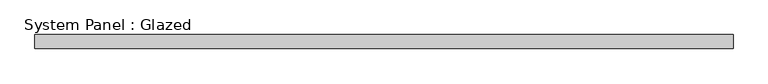
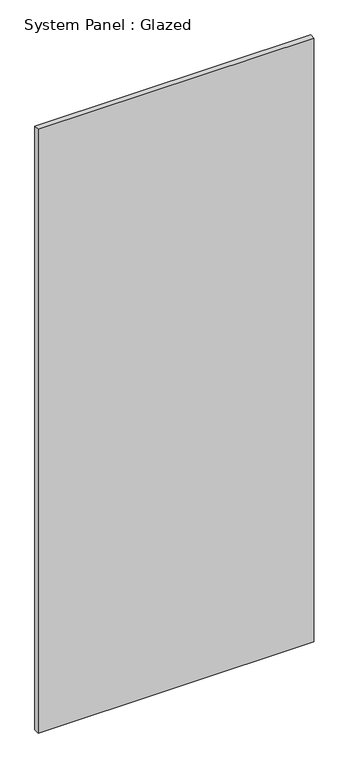
"""IFC4 building model written with IfcOpenShell, lengths in millimetres: plate geometry, System Panel : Glazed."""

from ifc_helpers import new_model, si_unit, origin, origin_with_axes, place, context, project, spatial, polyline, outline, extrude, source, transform, mapped, element, save


def system_panel_glazed_fd2dabf8(model_context):
    return source(origin(), model_context, "Body", "SweptSolid", [
        extrude(outline(polyline([(631.3526162, 19.05), (-631.3526162, 19.05), (-631.3526162, 44.45), (631.3526162, 44.45), (631.3526162, 19.05)])), origin_with_axes(), (0.0, 0.0, 1.0), 2921.0),
    ])


if __name__ == "__main__":
    model = new_model("IFC4")
    model_context = context("Model", 3, world=origin())
    ifc_project = project(units=[si_unit("LENGTHUNIT", "METRE", prefix="MILLI")], contexts=[model_context])
    site = spatial("IfcSite", under=ifc_project)
    building = spatial("IfcBuilding", under=site)
    placement = place(None, origin())
    system_panel_glazed_shape = system_panel_glazed_fd2dabf8(model_context)
    element("IfcPlate", 1, ObjectType="System Panel : Glazed", at=placement, inside=building, context=model_context, shape_type="MappedRepresentation", body=[
        mapped(system_panel_glazed_shape, transform((0.0, 0.0, 0.0), x_axis=(1.0, 0.0, 0.0), y_axis=(0.0, 1.0, 0.0), z_axis=(0.0, 0.0, 1.0))),
    ])
    save(model, "model.ifc")

# Revit data of these elements
# Type "System Panel : Glazed"
#   Construction Type Id = "GSP4R"
#   Analytic Construction = "1/8 in Pilkington single glazing"
#   Visual Light Transmittance = 0.9
#   Solar Heat Gain Coefficient = 0.86
#   Heat Transfer Coefficient (U) = 1.18115 BTU/(h·ft²·°F)
# Element 1 (IfcPlate, "System Panel : Glazed")
#   Materials on its faces: "Glass"
# Materials
#   "Glass": class "Glass", colour RGB 0 128 192, transparency 0.75, Description = "Soda Lime Glass", Cost = 0
